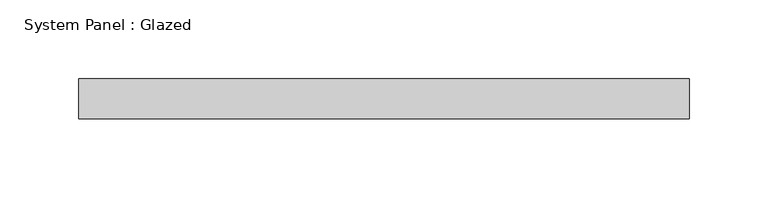
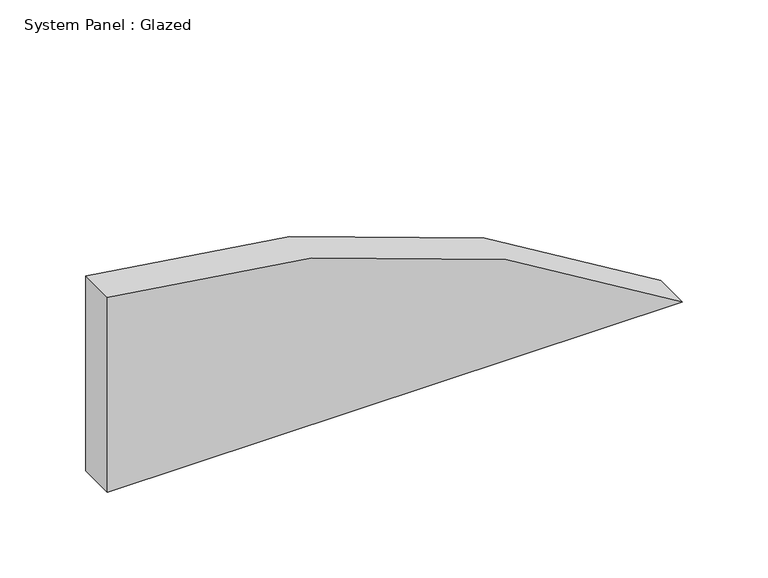
"""IFC4 building model written with IfcOpenShell, lengths in millimetres: plate geometry, System Panel : Glazed."""

from ifc_helpers import new_model, si_unit, point, frame, frame_2d, origin, place, context, project, spatial, polyline, circle_curve, trimmed, segment, composite_curve, outline, extrude, source, transform, mapped, element, save


def system_panel_glazed_ec3758d8(model_context):
    return source(origin(), model_context, "Body", "SweptSolid", [
        extrude(outline(composite_curve([segment(polyline([(0.0, -193.675), (0.0, 193.675)]), True, "CONTINUOUS"), segment(trimmed(circle_curve(frame_2d((-558.8, -225.425)), 698.5), [point((0.0, 193.675))], [point((138.978036, -193.675))], False, "CARTESIAN"), True, "CONTINUOUS"), segment(polyline([(138.978036, -193.675), (0.0, -193.675)]), True, "CONTINUOUS")], self_intersect=False)), frame((0.0, 19.05, 0.0), z_axis=(0.0, 1.0, 0.0), x_axis=(0.0, 0.0, 1.0)), (0.0, 0.0, 1.0), 25.4),
    ])


if __name__ == "__main__":
    model = new_model("IFC4")
    model_context = context("Model", 3, world=origin())
    ifc_project = project(units=[si_unit("LENGTHUNIT", "METRE", prefix="MILLI")], contexts=[model_context])
    site = spatial("IfcSite", under=ifc_project)
    building = spatial("IfcBuilding", under=site)
    placement = place(None, origin())
    system_panel_glazed_shape = system_panel_glazed_ec3758d8(model_context)
    element("IfcPlate", 1, ObjectType="System Panel : Glazed", at=placement, inside=building, context=model_context, shape_type="MappedRepresentation", body=[
        mapped(system_panel_glazed_shape, transform((0.0, 0.0, 0.0), x_axis=(1.0, 0.0, 0.0), y_axis=(0.0, 1.0, 0.0), z_axis=(0.0, 0.0, 1.0))),
    ])
    save(model, "model.ifc")

# Revit data of these elements
# Type "System Panel : Glazed"
#   Construction Type Id = "GSP4R"
#   Analytic Construction = "1/8 in Pilkington single glazing"
#   Visual Light Transmittance = 0.9
#   Solar Heat Gain Coefficient = 0.86
#   Heat Transfer Coefficient (U) = 1.18115 BTU/(h·ft²·°F)
#   Define Thermal Properties by = 1
# Element 1 (IfcPlate, "System Panel : Glazed")
#   Materials on its faces: "Glass"
# Materials
#   "Glass": class "Glass", colour RGB 0 128 192, transparency 0.75, Description = "Soda Lime Glass", Cost = 0
